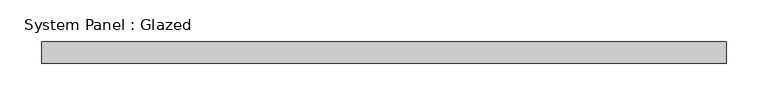
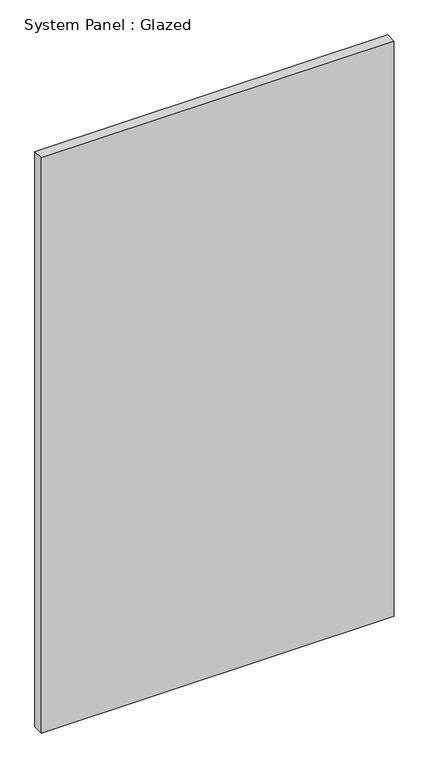
"""IFC4 building model written with IfcOpenShell, lengths in millimetres: plate geometry, System Panel : Glazed."""

from ifc_helpers import new_model, si_unit, origin, origin_with_axes, place, context, project, spatial, polyline, outline, extrude, source, transform, mapped, element, save


def system_panel_glazed_e7030ff9(model_context):
    return source(origin(), model_context, "Body", "SweptSolid", [
        extrude(outline(polyline([(409.575, 19.05), (-409.575, 19.05), (-409.575, 44.45), (409.575, 44.45), (409.575, 19.05)])), origin_with_axes(), (0.0, 0.0, 1.0), 1412.437083),
    ])


if __name__ == "__main__":
    model = new_model("IFC4")
    model_context = context("Model", 3, world=origin())
    ifc_project = project(units=[si_unit("LENGTHUNIT", "METRE", prefix="MILLI")], contexts=[model_context])
    site = spatial("IfcSite", under=ifc_project)
    building = spatial("IfcBuilding", under=site)
    placement = place(None, origin())
    system_panel_glazed_shape = system_panel_glazed_e7030ff9(model_context)
    element("IfcPlate", 1, ObjectType="System Panel : Glazed", at=placement, inside=building, context=model_context, shape_type="MappedRepresentation", body=[
        mapped(system_panel_glazed_shape, transform((0.0, 0.0, 0.0), x_axis=(1.0, 0.0, 0.0), y_axis=(0.0, 1.0, 0.0), z_axis=(0.0, 0.0, 1.0))),
    ])
    save(model, "model.ifc")

# Revit data of these elements
# Type "System Panel : Glazed"
#   Construction Type Id = "GSP4R"
#   Analytic Construction = "1/8 in Pilkington single glazing"
#   Visual Light Transmittance = 0.9
#   Solar Heat Gain Coefficient = 0.86
#   Heat Transfer Coefficient (U) = 1.18115 BTU/(h·ft²·°F)
#   Define Thermal Properties by = 1
# Element 1 (IfcPlate, "System Panel : Glazed")
#   Materials on its faces: "Glass"
# Materials
#   "Glass": class "Glass", colour RGB 0 128 192, transparency 0.75, Description = "Soda Lime Glass", Cost = 0
